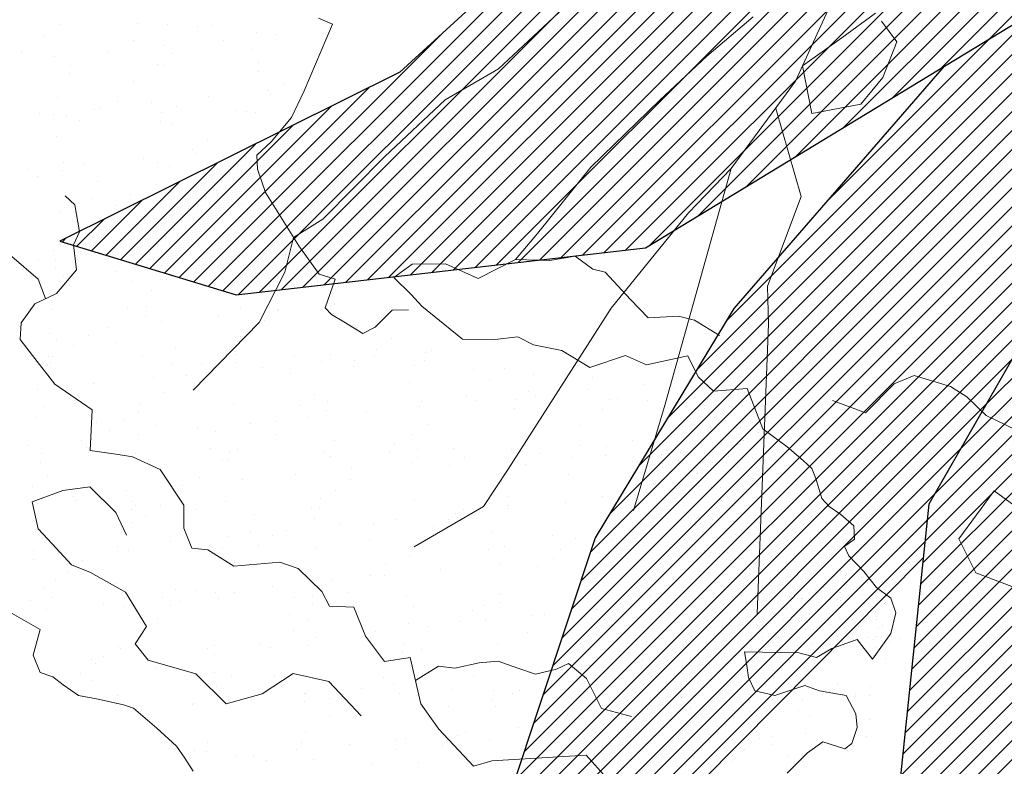
# Model space of a CAD drawing. Units: inches. Extents: x 1986 to 21484, y -1816 to 2016.
# Tile 55 of 85: x 3651.09 to 3662.33, y 1870.8 to 1879.32. Entities that reach past the tile are written whole.
import ezdxf

# ---------------------------------------------------------------- set-up
doc = ezdxf.new("R2010")
doc.units = ezdxf.units.IN
doc.layers.add('L-PLNT', color=84, linetype='Continuous', lineweight=13)
doc.layers.add('vfolhas', color=114, linetype='Continuous', lineweight=5)
for name, color, linetype in [('vfolha', 72, 'Continuous'), ('vfolha2', 110, 'Continuous'), ('vfolhas2', 102, 'Continuous')]:
    doc.layers.add(name, color=color, linetype=linetype)
pattern_1 = [(45, (-2446.5133113, 50.986076), (-0.004419417382, 0.004419417382), [])]

# ---------------------------------------------------------------- blocks, each defined once
blk = doc.blocks.new('arbusto_PB_verde_grande')
at = {"layer": 'vfolha2'}
h = blk.add_hatch(dxfattribs=at)
h.set_pattern_fill('ANSI31', color=256, scale=0.05, style=0)
h.set_pattern_definition(pattern_1)
h.paths.add_polyline_path([(0.02944, 0.35651), (0.00028, 0.09048), (0.02625, -0.03934), (0.047, 0.06233), (0.06189, 0.09731), (0.09372, 0.26573), (0.09955, 0.43473), (0.08789, 0.61313), (0.0645, 0.72266), (0.04988, 0.6851), (0.0236, 0.51294)])
h.paths.add_polyline_path([(0.30106, 0.43789), (0.14225, 0.24871), (0.26685, 0.30022)])
h.paths.add_polyline_path([(0.37995, 0.22817), (0.23697, 0.15193), (0.18428, 0.09364), (0.11122, 0.04358), (0.02625, -0.03934), (0.28061, 0.04667), (0.36829, 0.07798), (0.46756, 0.11239), (0.61068, 0.19376), (0.71585, 0.27823), (0.55813, 0.25948)])
h.paths.add_polyline_path([(0.56101, -0.29441), (0.72752, -0.32573), (0.59024, -0.2412), (0.42962, -0.15982), (0.02625, -0.03934), (0.14922, -0.14107), (0.18838, -0.16604), (0.41501, -0.24435)])
h.paths.add_polyline_path([(-0.27429, -0.44776), (-0.30352, -0.72628), (-0.23923, -0.64175), (-0.15457, -0.45716), (0.02625, -0.03934), (-0.16328, -0.25376)])
h.paths.add_polyline_path([(-0.51963, -0.24744), (-0.67736, -0.32573), (-0.59558, -0.35072), (-0.40574, -0.32882), (-0.21007, -0.20995), (0.02625, -0.03934), (-0.14874, -0.06595), (-0.31518, -0.09101), (-0.41452, -0.15048)])
h.paths.add_polyline_path([(-0.52546, 0.25007), (-0.70947, 0.24698), (-0.51963, 0.1093), (-0.32979, 0.02167), (-0.07567, -0.0128), (-0.04234, -0.02148), (-0.35024, 0.1312)])
at = {"layer": 'vfolhas'}
h = blk.add_hatch(dxfattribs=at)
h.set_pattern_fill('ANSI31', color=256, scale=0.05, style=0)
h.set_pattern_definition(pattern_1)
h.paths.add_polyline_path([(-0.57219, 0.06233), (-0.7153, 0.10298), (-0.67736, 0.08107), (-0.62769, 0.01536), (-0.56347, -0.04095), (-0.26461, -0.0834), (-0.14874, -0.06595), (-0.10151, -0.05877), (-0.20418, -0.0472), (-0.40279, -0.00339)])
h.paths.add_polyline_path([(-0.56347, -0.04095), (-0.58279, -0.02401), (-0.72992, -0.09726), (-0.4334, -0.1679), (-0.41452, -0.15048), (-0.31518, -0.09101), (-0.26461, -0.0834)])
h.paths.add_polyline_path([(-0.2769, -0.47267), (-0.27429, -0.44776), (-0.16328, -0.25376), (0.02625, -0.03934), (-0.21007, -0.20995), (-0.2672, -0.24466), (-0.36485, -0.35697), (-0.42907, -0.46341), (-0.47586, -0.60425), (-0.37946, -0.57603)])
at = {"layer": 'vfolha'}
blk.add_line((-0.2672, -0.24466), (-0.36485, -0.35697), dxfattribs=at)
at = {"layer": 'vfolha2'}
for p, q in [((-0.41452, -0.15048), (-0.51963, -0.24744)), ((-0.40574, -0.32882), (-0.21007, -0.20995)), ((-0.51963, -0.24744), (-0.67736, -0.32573)), ((-0.16328, -0.25376), (-0.27429, -0.44776)), ((-0.67736, -0.32573), (-0.59558, -0.35072)), ((-0.59558, -0.35072), (-0.40574, -0.32882)), ((-0.27429, -0.44776), (-0.30352, -0.72628))]:
    blk.add_line(p, q, dxfattribs=at)
at = {"layer": 'vfolhas2'}
for p, q in [((-0.36485, -0.35697), (-0.42907, -0.46341)), ((-0.42907, -0.46341), (-0.47586, -0.60425)), ((-0.37946, -0.57603), (-0.2769, -0.47267))]:
    blk.add_line(p, q, dxfattribs=at)
blk = doc.blocks.new('PLANT-SHRUB')
for p, q in [((2177.672, 1894.564), (2177.672, 1894.564)), ((2177.944, 1894.39), (2177.944, 1894.39)), ((2178.017, 1894.405), (2178.017, 1894.405)), ((2178.018, 1894.458), (2178.018, 1894.458)), ((2177.065, 1894.178), (2177.065, 1894.178)), ((2177.327, 1894.204), (2177.327, 1894.204)), ((2178.31, 1894.176), (2178.31, 1894.176)), ((2177.453, 1894.049), (2177.453, 1894.049)), ((2177.87, 1894.133), (2177.87, 1894.133)), ((2178.078, 1894.105), (2178.078, 1894.105)), ((2178.142, 1894.068), (2178.142, 1894.068)), ((2178.403, 1894.062), (2178.403, 1894.062)), ((2177.546, 1894.026), (2177.546, 1894.026)), ((2178.532, 1894.01), (2178.532, 1894.01)), ((2176.315, 1893.671), (2176.561, 1893.167)), ((2177.992, 1893.635), (2177.992, 1893.635)), ((2178.748, 1893.675), (2178.748, 1893.675)), ((2178.925, 1893.619), (2178.757, 1893.53)), ((2179.023, 1893.61), (2178.925, 1893.619)), ((2179.014, 1893.64), (2179.014, 1893.64)), ((2179.155, 1893.38), (2179.023, 1893.61)), ((2177.349, 1893.564), (2177.349, 1893.564)), ((2178.594, 1893.561), (2178.594, 1893.561)), ((2178.757, 1893.53), (2178.66, 1893.407)), ((2178.66, 1893.407), (2178.598, 1893.177)), ((2179.368, 1893.353), (2179.155, 1893.38)), ((2179.695, 1893.362), (2179.368, 1893.353)), ((2177.427, 1893.279), (2177.427, 1893.279)), ((2178.326, 1893.289), (2178.326, 1893.289)), ((2178.4, 1893.356), (2178.4, 1893.356)), ((2176.561, 1893.167), (2176.438, 1892.753)), ((2177.502, 1893.146), (2177.502, 1893.146)), ((2177.987, 1893.175), (2177.987, 1893.175)), ((2178.507, 1893.24), (2178.507, 1893.24)), ((2178.598, 1893.177), (2178.784, 1892.929)), ((2179.232, 1893.173), (2179.232, 1893.173)), ((2179.553, 1893.226), (2179.553, 1893.226)), ((2175.766, 1892.63), (2175.688, 1893.055)), ((2177.71, 1893.119), (2177.71, 1893.119)), ((2178.094, 1893.079), (2177.74, 1893.009)), ((2177.819, 1893.067), (2177.819, 1893.067)), ((2178.035, 1893.076), (2178.035, 1893.076)), ((2178.053, 1893.059), (2178.053, 1893.059)), ((2178.067, 1892.797), (2178.094, 1893.079)), ((2178.094, 1893.079), (2178.094, 1893.079)), ((2179.063, 1893.065), (2179.063, 1893.065)), ((2177.74, 1893.009), (2177.537, 1892.876)), ((2177.894, 1892.913), (2177.894, 1892.913)), ((2177.929, 1892.924), (2177.929, 1892.924)), ((2177.973, 1893.018), (2177.973, 1893.018)), ((2178.578, 1893.005), (2178.578, 1893.005)), ((2178.784, 1892.929), (2178.864, 1892.77)), ((2178.786, 1892.977), (2178.786, 1892.977)), ((2179.111, 1892.935), (2179.111, 1892.935)), ((2179.528, 1892.938), (2179.528, 1892.938)), ((2179.602, 1893.005), (2179.602, 1893.005)), ((2177.537, 1892.876), (2177.466, 1892.717)), ((2177.748, 1892.875), (2177.748, 1892.875)), ((2177.797, 1892.866), (2177.797, 1892.866)), ((2177.966, 1892.865), (2177.966, 1892.865)), ((2178.989, 1892.87), (2178.989, 1892.87)), ((2179.653, 1892.863), (2179.653, 1892.863)), ((2179.862, 1892.836), (2179.862, 1892.836)), ((2180.068, 1892.831), (2180.068, 1892.831)), ((2176.438, 1892.753), (2175.766, 1892.63)), ((2177.466, 1892.717), (2177.501, 1892.514)), ((2177.479, 1892.735), (2177.479, 1892.735)), ((2177.545, 1892.715), (2177.545, 1892.715)), ((2177.554, 1892.711), (2177.554, 1892.711)), ((2177.562, 1892.724), (2177.562, 1892.724)), ((2177.692, 1892.707), (2177.692, 1892.707)), ((2177.726, 1892.758), (2177.726, 1892.758)), ((2177.755, 1892.785), (2177.755, 1892.785)), ((2177.963, 1892.71), (2177.963, 1892.71)), ((2178.052, 1892.71), (2178.052, 1892.71)), ((2178.35, 1892.673), (2178.067, 1892.797)), ((2178.864, 1892.77), (2179.191, 1892.62)), ((2177.487, 1892.668), (2177.487, 1892.668)), ((2177.567, 1892.613), (2177.567, 1892.613)), ((2177.581, 1892.606), (2177.581, 1892.606)), ((2177.91, 1892.679), (2177.91, 1892.679)), ((2177.985, 1892.667), (2177.985, 1892.667)), ((2177.993, 1892.668), (2177.993, 1892.668)), ((2178.123, 1892.651), (2178.123, 1892.651)), ((2178.206, 1892.618), (2178.206, 1892.618)), ((2178.236, 1892.645), (2178.236, 1892.645)), ((2178.34, 1892.622), (2178.34, 1892.622)), ((2178.545, 1892.629), (2178.35, 1892.673)), ((2178.423, 1892.611), (2178.423, 1892.611)), ((2178.66, 1892.452), (2178.545, 1892.629)), ((2178.553, 1892.594), (2178.553, 1892.594)), ((2179.13, 1892.573), (2179.13, 1892.573)), ((2179.191, 1892.62), (2179.323, 1892.425)), ((2177.027, 1892.563), (2177.027, 1892.563)), ((2177.402, 1892.509), (2177.402, 1892.509)), ((2177.501, 1892.514), (2177.484, 1892.284)), ((2177.507, 1892.538), (2177.507, 1892.538)), ((2177.668, 1892.465), (2177.668, 1892.465)), ((2177.738, 1892.567), (2177.738, 1892.567)), ((2178.047, 1892.472), (2178.047, 1892.472)), ((2178.166, 1892.464), (2178.166, 1892.464)), ((2178.169, 1892.551), (2178.169, 1892.551)), ((2178.271, 1892.561), (2178.271, 1892.561)), ((2178.482, 1892.47), (2178.482, 1892.47)), ((2178.588, 1892.546), (2178.588, 1892.546)), ((2179.516, 1892.558), (2179.516, 1892.558)), ((2175.047, 1892.46), (2175.244, 1891.941)), ((2177.535, 1892.407), (2177.535, 1892.407)), ((2177.953, 1892.402), (2177.953, 1892.402)), ((2178.362, 1892.404), (2178.362, 1892.404)), ((2179.102, 1892.019), (2178.66, 1892.452)), ((2179.323, 1892.425), (2179.27, 1892.266)), ((2179.528, 1892.456), (2179.528, 1892.456)), ((2177.484, 1892.284), (2177.484, 1892.037)), ((2177.545, 1892.313), (2177.545, 1892.313)), ((2177.727, 1892.259), (2177.727, 1892.259)), ((2177.762, 1892.284), (2177.762, 1892.284)), ((2177.845, 1892.273), (2177.845, 1892.273)), ((2177.855, 1892.267), (2177.855, 1892.267)), ((2177.879, 1892.318), (2177.879, 1892.318)), ((2177.908, 1892.345), (2177.908, 1892.345)), ((2177.923, 1892.31), (2177.923, 1892.31)), ((2177.975, 1892.256), (2177.975, 1892.256)), ((2178.159, 1892.243), (2178.159, 1892.243)), ((2178.353, 1892.266), (2178.353, 1892.266)), ((2178.421, 1892.309), (2178.421, 1892.309)), ((2178.528, 1892.332), (2178.528, 1892.332)), ((2178.578, 1892.238), (2178.578, 1892.238)), ((2178.782, 1892.255), (2178.782, 1892.255)), ((2179.27, 1892.266), (2179.191, 1892.151)), ((2177.665, 1892.174), (2177.665, 1892.174)), ((2177.719, 1892.172), (2177.719, 1892.172)), ((2178.193, 1892.228), (2178.193, 1892.228)), ((2178.276, 1892.217), (2178.276, 1892.217)), ((2178.359, 1892.178), (2178.359, 1892.178)), ((2178.389, 1892.205), (2178.389, 1892.205)), ((2178.406, 1892.199), (2178.406, 1892.199)), ((2178.623, 1892.171), (2178.623, 1892.171)), ((2178.706, 1892.16), (2178.706, 1892.16)), ((2178.709, 1892.187), (2178.709, 1892.187)), ((2178.836, 1892.143), (2178.836, 1892.143)), ((2178.909, 1892.172), (2178.909, 1892.172)), ((2179.191, 1892.151), (2179.102, 1892.019)), ((2180.154, 1892.169), (2180.154, 1892.169)), ((2180.332, 1892.223), (2180.332, 1892.223)), ((2177.484, 1892.037), (2177.448, 1891.922)), ((2177.666, 1892.09), (2177.666, 1892.09)), ((2177.941, 1892.095), (2177.941, 1892.095)), ((2177.943, 1892.094), (2177.943, 1892.094)), ((2178.036, 1892.064), (2178.036, 1892.064)), ((2178.2, 1892.032), (2178.2, 1892.032)), ((2178.209, 1892.018), (2178.209, 1892.018)), ((2178.352, 1892.096), (2178.352, 1892.096)), ((2178.534, 1892.063), (2178.534, 1892.063)), ((2178.741, 1892.064), (2178.741, 1892.064)), ((2178.784, 1892.08), (2178.784, 1892.08)), ((2178.84, 1892.037), (2178.84, 1892.037)), ((2178.869, 1892.064), (2178.869, 1892.064)), ((2178.964, 1892.1), (2178.964, 1892.1)), ((2179.032, 1892.062), (2179.032, 1892.062)), ((2179.102, 1892.019), (2179.102, 1892.019)), ((2179.985, 1892.062), (2179.985, 1892.062)), ((2180.043, 1892.061), (2180.043, 1892.061)), ((2175.244, 1891.941), (2175.262, 1891.636)), ((2177.307, 1891.939), (2177.209, 1891.824)), ((2177.448, 1891.922), (2177.307, 1891.939)), ((2178.292, 1891.909), (2178.292, 1891.909)), ((2178.417, 1891.991), (2178.417, 1891.991)), ((2178.568, 1891.93), (2178.568, 1891.93)), ((2178.742, 1891.948), (2178.742, 1891.948)), ((2178.789, 1891.908), (2178.789, 1891.908)), ((2179.984, 1891.904), (2179.984, 1891.904)), ((2181.234, 1891.991), (2181.225, 1891.643)), ((2176.344, 1889.483), (2178.697, 1891.799)), ((2177.209, 1891.824), (2177.227, 1891.63)), ((2178.681, 1891.891), (2178.681, 1891.891)), ((2178.722, 1891.865), (2178.722, 1891.865)), ((2179.285, 1891.877), (2179.285, 1891.877)), ((2179.493, 1891.849), (2179.493, 1891.849)), ((2179.818, 1891.807), (2179.818, 1891.807)), ((2179.91, 1891.837), (2179.91, 1891.837)), ((2178.689, 1891.748), (2178.689, 1891.748)), ((2179.503, 1891.686), (2179.503, 1891.686)), ((2180.361, 1891.735), (2180.361, 1891.735)), ((2180.525, 1891.691), (2180.525, 1891.691)), ((2180.736, 1891.375), (2180.547, 1891.676)), ((2180.569, 1891.708), (2180.569, 1891.708)), ((2175.262, 1891.636), (2175.316, 1891.422)), ((2177.227, 1891.63), (2177.262, 1891.471)), ((2178.558, 1891.622), (2178.558, 1891.622)), ((2180.894, 1891.665), (2180.894, 1891.665)), ((2181.225, 1891.643), (2182.057, 1890.952)), ((2181.437, 1891.593), (2181.437, 1891.593)), ((2177.262, 1891.471), (2177.262, 1891.347)), ((2178.593, 1891.464), (2178.593, 1891.464)), ((2178.66, 1891.507), (2178.66, 1891.507)), ((2178.764, 1891.464), (2178.764, 1891.464)), ((2179.193, 1891.557), (2179.193, 1891.557)), ((2179.512, 1891.472), (2179.512, 1891.472)), ((2180.438, 1891.555), (2180.438, 1891.555)), ((2181.112, 1891.486), (2181.112, 1891.486)), ((2181.185, 1891.553), (2181.185, 1891.553)), ((2175.316, 1891.422), (2175.531, 1891.046)), ((2177.262, 1891.347), (2177.156, 1891.135)), ((2178.328, 1891.382), (2178.328, 1891.382)), ((2178.411, 1891.371), (2178.411, 1891.371)), ((2178.541, 1891.354), (2178.541, 1891.354)), ((2180.625, 1891.008), (2180.736, 1891.375)), ((2178.276, 1891.262), (2178.276, 1891.262)), ((2178.548, 1891.314), (2178.548, 1891.314)), ((2178.665, 1891.296), (2178.665, 1891.296)), ((2178.694, 1891.323), (2178.694, 1891.323)), ((2178.758, 1891.325), (2178.758, 1891.325)), ((2178.938, 1891.33), (2178.938, 1891.33)), ((2180.018, 1891.291), (2180.018, 1891.291)), ((2181.064, 1891.278), (2181.064, 1891.278)), ((2177.156, 1891.135), (2177.112, 1891.02)), ((2178.322, 1891.171), (2178.322, 1891.171)), ((2178.506, 1891.151), (2178.506, 1891.151)), ((2179.165, 1891.153), (2179.165, 1891.153)), ((2179.831, 1891.169), (2179.831, 1891.169)), ((2180.714, 1891.121), (2180.714, 1891.121)), ((2181.076, 1891.166), (2181.076, 1891.166)), ((2175.531, 1891.046), (2175.764, 1890.957)), ((2177.112, 1891.02), (2177.121, 1890.887)), ((2177.963, 1891.016), (2177.963, 1891.016)), ((2177.966, 1891.065), (2177.966, 1891.065)), ((2178.033, 1891.108), (2178.033, 1891.108)), ((2178.119, 1891.011), (2178.119, 1891.011)), ((2178.367, 1891.023), (2178.367, 1891.023)), ((2178.464, 1891.064), (2178.464, 1891.064)), ((2178.531, 1891.107), (2178.531, 1891.107)), ((2178.537, 1891.006), (2178.537, 1891.006)), ((2179.091, 1891.086), (2179.091, 1891.086)), ((2179.662, 1891.061), (2179.662, 1891.061)), ((2180.658, 1890.74), (2180.625, 1891.008)), ((2180.907, 1891.059), (2180.907, 1891.059)), ((2175.764, 1890.957), (2176.229, 1890.974)), ((2176.229, 1890.974), (2176.408, 1890.617)), ((2176.229, 1890.974), (2176.229, 1890.974)), ((2177.121, 1890.887), (2177.147, 1890.649)), ((2178.181, 1890.987), (2178.181, 1890.987)), ((2178.264, 1890.976), (2178.264, 1890.976)), ((2178.337, 1890.996), (2178.337, 1890.996)), ((2178.394, 1890.959), (2178.394, 1890.959)), ((2178.611, 1890.931), (2178.611, 1890.931)), ((2178.916, 1890.89), (2178.916, 1890.89)), ((2179.477, 1890.916), (2179.477, 1890.916)), ((2180.5, 1890.921), (2180.5, 1890.921)), ((2182.057, 1890.952), (2182.25, 1890.855)), ((2177.903, 1890.861), (2177.903, 1890.861)), ((2178.147, 1890.862), (2178.147, 1890.862)), ((2178.178, 1890.85), (2178.178, 1890.85)), ((2178.312, 1890.863), (2178.312, 1890.863)), ((2178.645, 1890.861), (2178.645, 1890.861)), ((2179.125, 1890.863), (2179.125, 1890.863)), ((2179.449, 1890.82), (2179.449, 1890.82)), ((2180.366, 1890.803), (2180.366, 1890.803)), ((2181.579, 1890.882), (2181.579, 1890.882)), ((2182.25, 1890.855), (2182.25, 1890.276)), ((2177.677, 1890.719), (2177.677, 1890.719)), ((2177.837, 1890.665), (2177.837, 1890.665)), ((2177.904, 1890.708), (2177.904, 1890.708)), ((2178.01, 1890.696), (2178.01, 1890.696)), ((2178.039, 1890.723), (2178.039, 1890.723)), ((2178.109, 1890.703), (2178.109, 1890.703)), ((2178.335, 1890.664), (2178.335, 1890.664)), ((2178.402, 1890.707), (2178.402, 1890.707)), ((2178.527, 1890.698), (2178.527, 1890.698)), ((2178.693, 1890.721), (2178.693, 1890.721)), ((2179.992, 1890.749), (2179.992, 1890.749)), ((2180.2, 1890.721), (2180.2, 1890.721)), ((2180.292, 1890.735), (2180.292, 1890.735)), ((2180.525, 1890.679), (2180.525, 1890.679)), ((2180.803, 1890.696), (2180.658, 1890.74)), ((2181.015, 1890.573), (2180.803, 1890.696)), ((2181.915, 1890.77), (2181.915, 1890.77)), ((2177.147, 1890.649), (2177.209, 1890.308)), ((2177.474, 1890.559), (2177.474, 1890.559)), ((2177.603, 1890.649), (2177.603, 1890.649)), ((2177.686, 1890.639), (2177.686, 1890.639)), ((2177.816, 1890.621), (2177.816, 1890.621)), ((2177.851, 1890.55), (2177.851, 1890.55)), ((2177.893, 1890.553), (2177.893, 1890.553)), ((2178.033, 1890.593), (2178.033, 1890.593)), ((2178.116, 1890.582), (2178.116, 1890.582)), ((2178.246, 1890.565), (2178.246, 1890.565)), ((2178.302, 1890.555), (2178.302, 1890.555)), ((2178.49, 1890.556), (2178.49, 1890.556)), ((2178.52, 1890.583), (2178.52, 1890.583)), ((2178.87, 1890.557), (2178.87, 1890.557)), ((2178.913, 1890.56), (2178.913, 1890.56)), ((2180.115, 1890.554), (2180.115, 1890.554)), ((2181.115, 1890.384), (2181.015, 1890.573)), ((2181.068, 1890.607), (2181.068, 1890.607)), ((2181.276, 1890.58), (2181.276, 1890.58)), ((2181.36, 1890.552), (2181.36, 1890.552)), ((2177.52, 1890.463), (2177.52, 1890.463)), ((2178.018, 1890.462), (2178.018, 1890.462)), ((2178.464, 1890.536), (2178.464, 1890.536)), ((2178.516, 1890.461), (2178.516, 1890.461)), ((2178.547, 1890.525), (2178.547, 1890.525)), ((2179.993, 1890.521), (2179.993, 1890.521)), ((2181.039, 1890.507), (2181.039, 1890.507)), ((2181.568, 1890.452), (2181.568, 1890.452)), ((2181.601, 1890.537), (2181.601, 1890.537)), ((2182.061, 1890.512), (2182.061, 1890.512)), ((2182.144, 1890.466), (2182.144, 1890.466)), ((2182.352, 1890.438), (2182.352, 1890.438)), ((2177.667, 1890.411), (2177.667, 1890.411)), ((2177.682, 1890.396), (2177.682, 1890.396)), ((2177.711, 1890.423), (2177.711, 1890.423)), ((2178.099, 1890.395), (2178.099, 1890.395)), ((2178.331, 1890.41), (2178.331, 1890.41)), ((2178.517, 1890.39), (2178.517, 1890.39)), ((2179.895, 1890.371), (2179.895, 1890.371)), ((2181.226, 1890.172), (2181.115, 1890.384)), ((2181.494, 1890.384), (2181.494, 1890.384)), ((2182.677, 1890.395), (2182.677, 1890.395)), ((2177.209, 1890.308), (2177.023, 1889.848)), ((2177.21, 1890.265), (2177.21, 1890.265)), ((2177.238, 1890.284), (2177.238, 1890.284)), ((2177.277, 1890.308), (2177.277, 1890.308)), ((2177.456, 1890.255), (2177.456, 1890.255)), ((2177.464, 1890.251), (2177.464, 1890.251)), ((2177.523, 1890.25), (2177.523, 1890.25)), ((2177.539, 1890.244), (2177.539, 1890.244)), ((2177.669, 1890.227), (2177.669, 1890.227)), ((2177.708, 1890.264), (2177.708, 1890.264)), ((2177.775, 1890.307), (2177.775, 1890.307)), ((2177.883, 1890.245), (2177.883, 1890.245)), ((2178.163, 1890.255), (2178.163, 1890.255)), ((2178.192, 1890.282), (2178.192, 1890.282)), ((2178.206, 1890.263), (2178.206, 1890.263)), ((2178.273, 1890.306), (2178.273, 1890.306)), ((2178.292, 1890.247), (2178.292, 1890.247)), ((2182.25, 1890.276), (2182.202, 1889.922)), ((2182.25, 1890.276), (2182.25, 1890.276)), ((2177.248, 1890.101), (2177.248, 1890.101)), ((2177.384, 1890.122), (2177.384, 1890.122)), ((2177.657, 1890.103), (2177.657, 1890.103)), ((2177.886, 1890.198), (2177.886, 1890.198)), ((2177.969, 1890.187), (2177.969, 1890.187)), ((2178.003, 1890.109), (2178.003, 1890.109)), ((2178.099, 1890.17), (2178.099, 1890.17)), ((2178.316, 1890.142), (2178.316, 1890.142)), ((2178.399, 1890.131), (2178.399, 1890.131)), ((2179.452, 1890.146), (2179.452, 1890.146)), ((2179.508, 1890.168), (2179.508, 1890.168)), ((2180.475, 1890.151), (2180.475, 1890.151)), ((2180.753, 1890.166), (2180.753, 1890.166)), ((2181.394, 1890.039), (2181.226, 1890.172)), ((2181.554, 1890.112), (2181.554, 1890.112)), ((2181.997, 1890.163), (2181.997, 1890.163)), ((2182.769, 1890.101), (2182.769, 1890.101)), ((2177.354, 1890.095), (2177.354, 1890.095)), ((2177.391, 1890.062), (2177.391, 1890.062)), ((2177.889, 1890.061), (2177.889, 1890.061)), ((2178.089, 1890.087), (2178.089, 1890.087)), ((2178.387, 1890.061), (2178.387, 1890.061)), ((2179.34, 1890.06), (2179.34, 1890.06)), ((2179.547, 1890.052), (2179.547, 1890.052)), ((2180.584, 1890.058), (2180.584, 1890.058)), ((2181.096, 1890.02), (2181.096, 1890.02)), ((2181.639, 1889.894), (2181.394, 1890.039)), ((2181.829, 1890.056), (2181.829, 1890.056)), ((2182.6, 1890.099), (2182.6, 1890.099)), ((2182.695, 1890.034), (2182.695, 1890.034)), ((2183.074, 1890.054), (2183.074, 1890.054)), ((2177.091, 1889.889), (2177.091, 1889.889)), ((2177.148, 1889.908), (2177.148, 1889.908)), ((2177.195, 1889.95), (2177.195, 1889.95)), ((2177.454, 1889.943), (2177.454, 1889.943)), ((2177.646, 1889.907), (2177.646, 1889.907)), ((2177.827, 1889.339), (2178.923, 1889.978)), ((2177.835, 1889.955), (2177.835, 1889.955)), ((2177.864, 1889.982), (2177.864, 1889.982)), ((2177.873, 1889.937), (2177.873, 1889.937)), ((2178.144, 1889.906), (2178.144, 1889.906)), ((2178.282, 1889.939), (2178.282, 1889.939)), ((2178.548, 1889.904), (2178.548, 1889.904)), ((2178.756, 1889.877), (2178.756, 1889.877)), ((2179.473, 1889.984), (2179.473, 1889.984)), ((2181.761, 1889.749), (2181.639, 1889.894)), ((2182.202, 1889.922), (2181.928, 1889.454)), ((2177.023, 1889.848), (2177.324, 1889.61)), ((2177.056, 1889.822), (2177.056, 1889.822)), ((2177.081, 1889.865), (2177.081, 1889.865)), ((2177.238, 1889.793), (2177.238, 1889.793)), ((2177.308, 1889.86), (2177.308, 1889.86)), ((2177.391, 1889.849), (2177.391, 1889.849)), ((2177.521, 1889.832), (2177.521, 1889.832)), ((2177.866, 1889.785), (2177.866, 1889.785)), ((2178.077, 1889.863), (2178.077, 1889.863)), ((2178.079, 1889.779), (2178.079, 1889.779)), ((2178.316, 1889.815), (2178.316, 1889.815)), ((2178.345, 1889.842), (2178.345, 1889.842)), ((2178.888, 1889.79), (2178.888, 1889.79)), ((2179.081, 1889.834), (2179.081, 1889.834)), ((2177.262, 1889.662), (2177.262, 1889.662)), ((2177.507, 1889.655), (2177.507, 1889.655)), ((2177.537, 1889.682), (2177.537, 1889.682)), ((2178.169, 1889.747), (2178.169, 1889.747)), ((2178.252, 1889.736), (2178.252, 1889.736)), ((2178.382, 1889.719), (2178.382, 1889.719)), ((2179.624, 1889.763), (2179.624, 1889.763)), ((2179.832, 1889.735), (2179.832, 1889.735)), ((2179.968, 1889.751), (2179.968, 1889.751)), ((2180.157, 1889.692), (2180.157, 1889.692)), ((2180.748, 1889.701), (2180.748, 1889.701)), ((2181.014, 1889.737), (2181.014, 1889.737)), ((2182.065, 1889.688), (2181.761, 1889.749)), ((2182.036, 1889.742), (2182.036, 1889.742)), ((2182.298, 1889.669), (2182.298, 1889.669)), ((2183.116, 1889.703), (2183.116, 1889.703)), ((2177.324, 1889.61), (2177.341, 1889.371)), ((2177.444, 1889.635), (2177.444, 1889.635)), ((2178.548, 1889.556), (2178.548, 1889.556)), ((2179.075, 1889.62), (2179.075, 1889.62)), ((2179.792, 1889.554), (2179.792, 1889.554)), ((2180.675, 1889.634), (2180.675, 1889.634)), ((2180.7, 1889.621), (2180.7, 1889.621)), ((2180.908, 1889.593), (2180.908, 1889.593)), ((2181.037, 1889.551), (2181.037, 1889.551)), ((2181.233, 1889.551), (2181.233, 1889.551)), ((2182.281, 1889.549), (2182.281, 1889.549)), ((2182.792, 1889.56), (2182.792, 1889.018)), ((2183.526, 1889.547), (2183.526, 1889.547)), ((2176.055, 1889.155), (2176.344, 1889.483)), ((2177.348, 1889.509), (2177.348, 1889.509)), ((2177.374, 1889.438), (2177.374, 1889.438)), ((2177.45, 1889.464), (2177.45, 1889.464)), ((2177.517, 1889.507), (2177.517, 1889.507)), ((2177.637, 1889.487), (2177.637, 1889.487)), ((2181.775, 1889.479), (2181.775, 1889.479)), ((2181.928, 1889.454), (2182.173, 1889.288)), ((2181.983, 1889.452), (2181.983, 1889.452)), ((2175.438, 1887.895), (2177.827, 1889.339)), ((2177.341, 1889.371), (2177.262, 1889.115)), ((2177.434, 1889.327), (2177.434, 1889.327)), ((2177.591, 1889.409), (2177.591, 1889.409)), ((2177.674, 1889.398), (2177.674, 1889.398)), ((2178.381, 1889.389), (2178.381, 1889.389)), ((2179.427, 1889.376), (2179.427, 1889.376)), ((2180.449, 1889.381), (2180.449, 1889.381)), ((2181.529, 1889.342), (2181.529, 1889.342)), ((2181.95, 1889.35), (2181.95, 1889.35)), ((2182.308, 1889.409), (2182.308, 1889.409)), ((2182.575, 1889.329), (2182.575, 1889.329)), ((2182.851, 1889.338), (2182.851, 1889.338)), ((2183.499, 1889.318), (2183.499, 1889.318)), ((2183.598, 1889.334), (2183.598, 1889.334)), ((2177.631, 1889.261), (2177.631, 1889.261)), ((2178.654, 1889.234), (2178.654, 1889.234)), ((2178.728, 1889.301), (2178.728, 1889.301)), ((2180.277, 1889.269), (2180.277, 1889.269)), ((2181.876, 1889.283), (2181.876, 1889.283)), ((2182.173, 1889.288), (2182.133, 1888.93)), ((2183.059, 1889.31), (2183.059, 1889.31)), ((2183.384, 1889.267), (2183.384, 1889.267)), ((2175.073, 1888.674), (2176.055, 1889.155)), ((2176.839, 1889.192), (2176.839, 1889.192)), ((2176.928, 1888.868), (2176.839, 1889.192)), ((2177.262, 1889.115), (2177.677, 1888.868)), ((2177.262, 1889.115), (2177.262, 1889.115)), ((2177.388, 1889.106), (2177.388, 1889.106)), ((2177.941, 1889.169), (2177.941, 1889.169)), ((2179.185, 1889.167), (2179.185, 1889.167)), ((2180.43, 1889.165), (2180.43, 1889.165)), ((2181.675, 1889.163), (2181.675, 1889.163)), ((2182.919, 1889.16), (2182.919, 1889.16)), ((2183.927, 1889.196), (2183.927, 1889.196)), ((2177.84, 1889.015), (2177.84, 1889.015)), ((2178.863, 1889.02), (2178.863, 1889.02)), ((2179.017, 1889.06), (2179.017, 1889.06)), ((2179.942, 1888.981), (2179.942, 1888.981)), ((2180.262, 1889.057), (2180.262, 1889.057)), ((2181.506, 1889.055), (2181.506, 1889.055)), ((2182.751, 1889.053), (2182.751, 1889.053)), ((2182.792, 1889.018), (2183.027, 1888.675)), ((2183.151, 1889), (2183.151, 1889)), ((2183.995, 1889.051), (2183.995, 1889.051)), ((2177.029, 1888.712), (2176.928, 1888.868)), ((2177.677, 1888.868), (2177.778, 1888.623)), ((2178.179, 1888.918), (2178.179, 1888.918)), ((2178.256, 1888.869), (2178.256, 1888.869)), ((2178.388, 1888.89), (2178.388, 1888.89)), ((2179.856, 1888.883), (2179.856, 1888.883)), ((2179.929, 1888.951), (2179.929, 1888.951)), ((2180.989, 1888.967), (2180.989, 1888.967)), ((2181.478, 1888.918), (2181.478, 1888.918)), ((2182.133, 1888.93), (2182.006, 1888.597)), ((2182.011, 1888.972), (2182.011, 1888.972)), ((2183.078, 1888.932), (2183.078, 1888.932)), ((2183.09, 1888.933), (2183.09, 1888.933)), ((2184.137, 1888.92), (2184.137, 1888.92)), ((2178.712, 1888.848), (2178.712, 1888.848)), ((2179.255, 1888.776), (2179.255, 1888.776)), ((2179.642, 1888.652), (2180.139, 1888.772)), ((2180.139, 1888.772), (2181.03, 1888.566)), ((2174.599, 1887.742), (2175.073, 1888.674)), ((2177.297, 1888.489), (2177.029, 1888.712)), ((2177.529, 1888.118), (2179.642, 1888.652)), ((2179.463, 1888.749), (2179.463, 1888.749)), ((2179.788, 1888.706), (2179.788, 1888.706)), ((2183.027, 1888.675), (2183.443, 1888.603)), ((2184.353, 1888.649), (2184.353, 1888.649)), ((2184.622, 1888.704), (2184.589, 1888.532)), ((2177.778, 1888.623), (2178.169, 1888.444)), ((2178.225, 1888.555), (2178.225, 1888.555)), ((2178.356, 1888.619), (2178.356, 1888.619)), ((2179.402, 1888.606), (2179.402, 1888.606)), ((2179.469, 1888.553), (2179.469, 1888.553)), ((2180.331, 1888.635), (2180.331, 1888.635)), ((2180.424, 1888.611), (2180.424, 1888.611)), ((2180.539, 1888.607), (2180.539, 1888.607)), ((2180.714, 1888.55), (2180.714, 1888.55)), ((2180.864, 1888.564), (2180.864, 1888.564)), ((2181.057, 1888.532), (2181.057, 1888.532)), ((2181.131, 1888.6), (2181.131, 1888.6)), ((2181.504, 1888.572), (2181.504, 1888.572)), ((2181.959, 1888.548), (2181.959, 1888.548)), ((2182.006, 1888.597), (2182.197, 1888.398)), ((2182.55, 1888.559), (2182.55, 1888.559)), ((2182.68, 1888.568), (2182.68, 1888.568)), ((2183.203, 1888.546), (2183.203, 1888.546)), ((2183.443, 1888.603), (2183.822, 1888.404)), ((2183.443, 1888.603), (2183.443, 1888.603)), ((2183.572, 1888.563), (2183.572, 1888.563)), ((2184.279, 1888.581), (2184.279, 1888.581)), ((2184.448, 1888.544), (2184.448, 1888.544)), ((2184.589, 1888.532), (2184.564, 1888.368)), ((2177.297, 1888.198), (2177.297, 1888.489)), ((2178.169, 1888.444), (2178.27, 1888.086)), ((2178.169, 1888.444), (2178.169, 1888.444)), ((2179.458, 1888.519), (2179.458, 1888.519)), ((2181.407, 1888.493), (2181.407, 1888.493)), ((2181.615, 1888.466), (2181.615, 1888.466)), ((2181.94, 1888.423), (2181.94, 1888.423)), ((2173.071, 1888.134), (2173.464, 1888.322)), ((2173.464, 1888.322), (2173.858, 1888.374)), ((2173.621, 1888.305), (2173.621, 1888.305)), ((2173.727, 1888.316), (2173.727, 1888.316)), ((2173.858, 1888.374), (2174.149, 1888.186)), ((2173.858, 1888.374), (2173.858, 1888.374)), ((2173.858, 1888.374), (2173.858, 1888.374)), ((2182.197, 1888.398), (2182.149, 1888.215)), ((2182.483, 1888.351), (2182.483, 1888.351)), ((2182.691, 1888.324), (2182.691, 1888.324)), ((2183.822, 1888.404), (2183.84, 1887.917)), ((2184.564, 1888.368), (2184.589, 1888.064)), ((2173.848, 1888.234), (2173.848, 1888.234)), ((2173.885, 1888.268), (2173.885, 1888.268)), ((2177.297, 1887.774), (2177.297, 1888.198)), ((2178.838, 1888.249), (2178.838, 1888.249)), ((2179.11, 1888.2), (2179.11, 1888.2)), ((2179.917, 1888.211), (2179.917, 1888.211)), ((2180.963, 1888.197), (2180.963, 1888.197)), ((2181.986, 1888.202), (2181.986, 1888.202)), ((2182.149, 1888.215), (2182.165, 1887.842)), ((2182.332, 1888.249), (2182.332, 1888.249)), ((2183.016, 1888.281), (2183.016, 1888.281)), ((2183.559, 1888.21), (2183.559, 1888.21)), ((2183.881, 1888.217), (2183.881, 1888.217)), ((2173.036, 1887.844), (2173.071, 1888.134)), ((2173.071, 1888.134), (2173.071, 1888.134)), ((2173.351, 1888.118), (2173.351, 1888.118)), ((2173.423, 1888.123), (2173.423, 1888.123)), ((2173.862, 1888.12), (2173.862, 1888.12)), ((2174.046, 1888.122), (2174.046, 1888.122)), ((2174.149, 1888.186), (2174.337, 1888.066)), ((2176.141, 1887.929), (2177.529, 1888.118)), ((2178.27, 1888.086), (2178.46, 1887.818)), ((2178.863, 1888.166), (2178.863, 1888.166)), ((2179.036, 1888.132), (2179.036, 1888.132)), ((2180.107, 1888.164), (2180.107, 1888.164)), ((2180.659, 1888.168), (2180.659, 1888.168)), ((2181.352, 1888.162), (2181.352, 1888.162)), ((2182.258, 1888.182), (2182.258, 1888.182)), ((2182.597, 1888.159), (2182.597, 1888.159)), ((2183.065, 1888.163), (2183.065, 1888.163)), ((2183.767, 1888.182), (2183.767, 1888.182)), ((2183.841, 1888.157), (2183.841, 1888.157)), ((2184.092, 1888.14), (2184.092, 1888.14)), ((2184.111, 1888.15), (2184.111, 1888.15)), ((2173.156, 1888.027), (2173.156, 1888.027)), ((2173.339, 1888.069), (2173.339, 1888.069)), ((2173.427, 1887.991), (2173.427, 1887.991)), ((2173.531, 1887.978), (2173.531, 1887.978)), ((2173.649, 1888.052), (2173.649, 1888.052)), ((2173.961, 1888.068), (2173.961, 1888.068)), ((2174.337, 1888.066), (2174.043, 1887.599)), ((2174.337, 1888.066), (2174.337, 1888.066)), ((2178.694, 1888.059), (2178.694, 1888.059)), ((2179.939, 1888.057), (2179.939, 1888.057)), ((2181.183, 1888.054), (2181.183, 1888.054)), ((2182.428, 1888.052), (2182.428, 1888.052)), ((2183.673, 1888.05), (2183.673, 1888.05)), ((2184.589, 1888.064), (2184.626, 1887.716)), ((2173.069, 1887.94), (2173.069, 1887.94)), ((2173.439, 1887.859), (2173.439, 1887.859)), ((2173.475, 1887.893), (2173.475, 1887.893)), ((2173.609, 1887.92), (2173.609, 1887.92)), ((2173.694, 1887.956), (2173.694, 1887.956)), ((2173.965, 1887.92), (2173.965, 1887.92)), ((2174.069, 1887.907), (2174.069, 1887.907)), ((2174.132, 1887.913), (2174.132, 1887.913)), ((2174.221, 1887.672), (2175.438, 1887.895)), ((2175.438, 1887.895), (2176.141, 1887.929)), ((2183.534, 1887.898), (2183.534, 1887.898)), ((2183.84, 1887.917), (2184.129, 1887.429)), ((2173.565, 1887.816), (2173.565, 1887.816)), ((2177.375, 1887.651), (2177.297, 1887.774)), ((2178.46, 1887.818), (2178.527, 1887.628)), ((2178.887, 1887.79), (2178.887, 1887.79)), ((2179.095, 1887.763), (2179.095, 1887.763)), ((2179.377, 1887.836), (2179.377, 1887.836)), ((2180.238, 1887.782), (2180.238, 1887.782)), ((2180.311, 1887.849), (2180.311, 1887.849)), ((2180.399, 1887.841), (2180.399, 1887.841)), ((2181.479, 1887.802), (2181.479, 1887.802)), ((2181.861, 1887.817), (2181.861, 1887.817)), ((2182.165, 1887.842), (2182.269, 1887.643)), ((2182.525, 1887.788), (2182.525, 1887.788)), ((2183.46, 1887.831), (2183.46, 1887.831)), ((2183.547, 1887.793), (2183.547, 1887.793)), ((2184.627, 1887.755), (2184.627, 1887.755)), ((2172.884, 1887.124), (2174.221, 1887.672)), ((2173.498, 1887.673), (2173.023, 1887.729)), ((2173.338, 1887.733), (2173.338, 1887.733)), ((2174.043, 1887.599), (2173.498, 1887.673)), ((2173.849, 1887.735), (2173.849, 1887.735)), ((2174.039, 1887.684), (2174.039, 1887.684)), ((2174.076, 1887.717), (2174.076, 1887.717)), ((2177.42, 1887.405), (2177.375, 1887.651)), ((2178.527, 1887.628), (2178.739, 1887.472)), ((2179.42, 1887.72), (2179.42, 1887.72)), ((2179.963, 1887.648), (2179.963, 1887.648)), ((2182.269, 1887.643), (2182.682, 1887.317)), ((2184.626, 1887.716), (2184.684, 1887.612)), ((2173.884, 1887.621), (2173.884, 1887.621)), ((2179.147, 1887.552), (2179.147, 1887.552)), ((2180.171, 1887.621), (2180.171, 1887.621)), ((2180.391, 1887.55), (2180.391, 1887.55)), ((2180.496, 1887.578), (2180.496, 1887.578)), ((2181.636, 1887.547), (2181.636, 1887.547)), ((2182.88, 1887.545), (2182.88, 1887.545)), ((2184.125, 1887.543), (2184.125, 1887.543)), ((2184.684, 1887.612), (2184.851, 1887.364)), ((2184.735, 1887.547), (2184.735, 1887.547)), ((2177.667, 1887.245), (2177.42, 1887.405)), ((2178.739, 1887.472), (2179.007, 1887.215)), ((2179.84, 1887.417), (2179.84, 1887.417)), ((2179.892, 1887.44), (2179.892, 1887.44)), ((2180.938, 1887.427), (2180.938, 1887.427)), ((2181.038, 1887.507), (2181.038, 1887.507)), ((2181.247, 1887.479), (2181.247, 1887.479)), ((2181.439, 1887.431), (2181.439, 1887.431)), ((2181.513, 1887.498), (2181.513, 1887.498)), ((2181.571, 1887.436), (2181.571, 1887.436)), ((2181.961, 1887.432), (2181.961, 1887.432)), ((2183.062, 1887.466), (2183.062, 1887.466)), ((2184.129, 1887.429), (2184.111, 1887.195)), ((2184.661, 1887.48), (2184.661, 1887.48)), ((2182.114, 1887.365), (2182.114, 1887.365)), ((2182.322, 1887.338), (2182.322, 1887.338)), ((2182.647, 1887.295), (2182.647, 1887.295)), ((2182.682, 1887.317), (2182.772, 1886.981)), ((2182.682, 1887.317), (2182.682, 1887.317)), ((2183.04, 1887.393), (2183.04, 1887.393)), ((2184.086, 1887.38), (2184.086, 1887.38)), ((2184.851, 1887.364), (2184.984, 1887.18)), ((2177.945, 1886.966), (2177.667, 1887.245)), ((2179.007, 1887.215), (2179.086, 1886.623)), ((2183.19, 1887.223), (2183.19, 1887.223)), ((2183.398, 1887.196), (2183.398, 1887.196)), ((2184.111, 1887.195), (2183.88, 1887.136)), ((2184.984, 1887.18), (2185.03, 1886.972)), ((2179.492, 1887.099), (2179.492, 1887.099)), ((2179.784, 1887.163), (2179.784, 1887.163)), ((2180.374, 1887.071), (2180.374, 1887.071)), ((2181.029, 1887.161), (2181.029, 1887.161)), ((2182.274, 1887.159), (2182.274, 1887.159)), ((2182.641, 1887.08), (2182.641, 1887.08)), ((2182.714, 1887.148), (2182.714, 1887.148)), ((2183.518, 1887.156), (2183.518, 1887.156)), ((2183.723, 1887.153), (2183.723, 1887.153)), ((2183.88, 1887.136), (2183.785, 1886.689)), ((2184.264, 1887.115), (2184.264, 1887.115)), ((2184.266, 1887.082), (2184.266, 1887.082)), ((2184.763, 1887.154), (2184.763, 1887.154)), ((2177.558, 1886.922), (2177.945, 1886.966)), ((2178.404, 1886.835), (2177.945, 1886.966)), ((2179.352, 1887.066), (2179.352, 1887.066)), ((2179.419, 1887.031), (2179.419, 1887.031)), ((2179.616, 1887.056), (2179.616, 1887.056)), ((2180.861, 1887.054), (2180.861, 1887.054)), ((2181.041, 1887.066), (2181.041, 1887.066)), ((2181.453, 1887.032), (2181.453, 1887.032)), ((2182.105, 1887.051), (2182.105, 1887.051)), ((2182.5, 1887.018), (2182.5, 1887.018)), ((2182.772, 1886.981), (2182.892, 1886.841)), ((2183.35, 1887.049), (2183.35, 1887.049)), ((2183.522, 1887.023), (2183.522, 1887.023)), ((2184.474, 1887.054), (2184.474, 1887.054)), ((2184.594, 1887.047), (2184.594, 1887.047)), ((2184.601, 1886.984), (2184.601, 1886.984)), ((2184.799, 1887.012), (2184.799, 1887.012)), ((2185.03, 1886.972), (2185.053, 1886.823)), ((2176.595, 1886.787), (2177.558, 1886.922)), ((2174.071, 1886.806), (2174.764, 1886.768)), ((2174.764, 1886.768), (2175.497, 1886.768)), ((2175.497, 1886.768), (2176.595, 1886.787)), ((2178.56, 1886.456), (2178.404, 1886.835)), ((2180.694, 1886.748), (2180.694, 1886.748)), ((2182.892, 1886.841), (2182.802, 1886.61)), ((2182.892, 1886.841), (2182.892, 1886.841)), ((2183.916, 1886.797), (2183.916, 1886.797)), ((2185.053, 1886.823), (2185.122, 1886.69)), ((2179.086, 1886.623), (2179.086, 1886.444)), ((2179.594, 1886.662), (2179.594, 1886.662)), ((2179.802, 1886.635), (2179.802, 1886.635)), ((2179.867, 1886.67), (2179.867, 1886.67)), ((2180.62, 1886.68), (2180.62, 1886.68)), ((2180.913, 1886.657), (2180.913, 1886.657)), ((2181.935, 1886.662), (2181.935, 1886.662)), ((2182.243, 1886.716), (2182.243, 1886.716)), ((2183.015, 1886.623), (2183.015, 1886.623)), ((2183.785, 1886.689), (2183.926, 1886.251)), ((2183.785, 1886.689), (2183.785, 1886.689)), ((2183.842, 1886.729), (2183.842, 1886.729)), ((2185.122, 1886.69), (2185.047, 1886.494)), ((2179.227, 1886.548), (2179.368, 1886.425)), ((2180.068, 1886.549), (2180.068, 1886.549)), ((2180.127, 1886.592), (2180.127, 1886.592)), ((2180.67, 1886.52), (2180.67, 1886.52)), ((2181.313, 1886.547), (2181.313, 1886.547)), ((2182.558, 1886.544), (2182.558, 1886.544)), ((2182.802, 1886.61), (2182.621, 1886.419)), ((2183.802, 1886.542), (2183.802, 1886.542)), ((2184.061, 1886.61), (2184.061, 1886.61)), ((2178.84, 1886.199), (2178.56, 1886.456)), ((2179.086, 1886.444), (2179.097, 1886.165)), ((2179.368, 1886.425), (2179.641, 1886.434)), ((2179.641, 1886.434), (2179.79, 1886.39)), ((2180.878, 1886.493), (2180.878, 1886.493)), ((2181.203, 1886.45), (2181.203, 1886.45)), ((2181.895, 1886.397), (2181.895, 1886.397)), ((2182.621, 1886.419), (2182.54, 1885.937)), ((2185.047, 1886.494), (2184.788, 1886.333)), ((2179.79, 1886.39), (2179.86, 1886.144)), ((2180.222, 1886.316), (2180.222, 1886.316)), ((2180.349, 1886.301), (2180.349, 1886.301)), ((2181.746, 1886.379), (2181.746, 1886.379)), ((2181.822, 1886.329), (2181.822, 1886.329)), ((2181.954, 1886.351), (2181.954, 1886.351)), ((2182.279, 1886.309), (2182.279, 1886.309)), ((2183.444, 1886.365), (2183.444, 1886.365)), ((2184.788, 1886.333), (2184.967, 1885.753)), ((2184.788, 1886.333), (2184.788, 1886.333)), ((2179.097, 1886.165), (2178.84, 1886.199)), ((2181.428, 1886.262), (2181.428, 1886.262)), ((2182.474, 1886.248), (2182.474, 1886.248)), ((2182.822, 1886.237), (2182.822, 1886.237)), ((2183.03, 1886.21), (2183.03, 1886.21)), ((2183.244, 1885.949), (2183.334, 1886.22)), ((2183.497, 1886.253), (2183.497, 1886.253)), ((2183.926, 1886.251), (2184.021, 1886.039)), ((2184.576, 1886.214), (2184.576, 1886.214)), ((2179.097, 1886.165), (2179.097, 1886.165)), ((2179.86, 1886.144), (2179.904, 1885.986)), ((2180.706, 1886.16), (2180.706, 1886.16)), ((2181.951, 1886.158), (2181.951, 1886.158)), ((2183.196, 1886.156), (2183.196, 1886.156)), ((2183.355, 1886.167), (2183.355, 1886.167)), ((2183.897, 1886.095), (2183.897, 1886.095)), ((2184.105, 1886.068), (2184.105, 1886.068)), ((2184.44, 1886.153), (2184.44, 1886.153)), ((2179.875, 1885.997), (2179.875, 1885.997)), ((2179.904, 1885.986), (2179.904, 1885.881)), ((2180.538, 1886.053), (2180.538, 1886.053)), ((2181.424, 1885.965), (2181.424, 1885.965)), ((2181.782, 1886.05), (2181.782, 1886.05)), ((2183.023, 1885.979), (2183.023, 1885.979)), ((2183.027, 1886.048), (2183.027, 1886.048)), ((2183.097, 1886.046), (2183.097, 1886.046)), ((2183.262, 1885.534), (2183.244, 1885.949)), ((2184.021, 1886.039), (2184.021, 1885.714)), ((2184.272, 1886.046), (2184.272, 1886.046)), ((2184.43, 1886.025), (2184.43, 1886.025)), ((2184.646, 1886.014), (2184.646, 1886.014)), ((2179.904, 1885.881), (2179.597, 1885.722)), ((2179.801, 1885.93), (2179.801, 1885.93)), ((2179.842, 1885.9), (2179.842, 1885.9)), ((2180.888, 1885.887), (2180.888, 1885.887)), ((2181.91, 1885.892), (2181.91, 1885.892)), ((2182.54, 1885.937), (2182.671, 1885.616)), ((2182.99, 1885.853), (2182.99, 1885.853)), ((2184.036, 1885.84), (2184.036, 1885.84)), ((2179.597, 1885.722), (2179.693, 1885.555)), ((2181.076, 1885.646), (2181.076, 1885.646)), ((2182.625, 1885.614), (2182.625, 1885.614)), ((2182.671, 1885.616), (2182.772, 1885.485)), ((2184.021, 1885.714), (2184.021, 1885.479)), ((2184.224, 1885.628), (2184.224, 1885.628)), ((2184.298, 1885.695), (2184.298, 1885.695)), ((2179.693, 1885.555), (2179.641, 1885.16)), ((2179.746, 1885.548), (2179.746, 1885.548)), ((2179.759, 1885.606), (2179.759, 1885.606)), ((2180.301, 1885.534), (2180.301, 1885.534)), ((2180.324, 1885.53), (2180.324, 1885.53)), ((2180.51, 1885.507), (2180.51, 1885.507)), ((2180.568, 1885.489), (2181.646, 1885.537)), ((2180.99, 1885.546), (2180.99, 1885.546)), ((2181.002, 1885.579), (2181.002, 1885.579)), ((2182.235, 1885.544), (2182.235, 1885.544)), ((2183.515, 1885.353), (2183.262, 1885.534)), ((2183.48, 1885.541), (2183.48, 1885.541)), ((2179.962, 1885.271), (2180.568, 1885.489)), ((2180.834, 1885.464), (2180.834, 1885.464)), ((2181.377, 1885.392), (2181.377, 1885.392)), ((2181.403, 1885.492), (2181.403, 1885.492)), ((2182.449, 1885.478), (2182.449, 1885.478)), ((2182.772, 1885.485), (2182.973, 1885.234)), ((2183.472, 1885.483), (2183.472, 1885.483)), ((2184.021, 1885.479), (2183.858, 1885.209)), ((2179.618, 1885.049), (2179.962, 1885.271)), ((2181.585, 1885.365), (2181.585, 1885.365)), ((2181.91, 1885.322), (2181.91, 1885.322)), ((2182.278, 1885.296), (2182.278, 1885.296)), ((2183.858, 1885.209), (2183.515, 1885.353)), ((2175.422, 1885.249), (2176.598, 1885.249)), ((2176.598, 1885.249), (2177.283, 1885.089)), ((2179.641, 1885.16), (2179.5, 1884.457)), ((2180.384, 1885.159), (2180.384, 1885.159)), ((2180.605, 1885.214), (2180.605, 1885.214)), ((2181.628, 1885.157), (2181.628, 1885.157)), ((2182.204, 1885.228), (2182.204, 1885.228)), ((2182.453, 1885.251), (2182.453, 1885.251)), ((2182.973, 1885.234), (2182.641, 1884.913)), ((2182.661, 1885.223), (2182.661, 1885.223)), ((2182.986, 1885.181), (2182.986, 1885.181)), ((2183.827, 1885.263), (2183.827, 1885.263)), ((2183.858, 1885.209), (2183.858, 1885.209)), ((2177.283, 1885.089), (2178.228, 1885.089)), ((2178.228, 1885.089), (2179.234, 1885.126)), ((2179.234, 1885.126), (2179.618, 1885.049)), ((2179.816, 1885.13), (2179.816, 1885.13)), ((2180.215, 1885.052), (2180.215, 1885.052)), ((2180.863, 1885.117), (2180.863, 1885.117)), ((2181.46, 1885.05), (2181.46, 1885.05)), ((2181.885, 1885.122), (2181.885, 1885.122)), ((2182.704, 1885.047), (2182.704, 1885.047)), ((2182.873, 1885.155), (2182.873, 1885.155)), ((2182.965, 1885.083), (2182.965, 1885.083)), ((2183.529, 1885.109), (2183.529, 1885.109)), ((2183.737, 1885.082), (2183.737, 1885.082)), ((2183.479, 1884.945), (2183.479, 1884.945)), ((2180.183, 1884.828), (2180.183, 1884.828)), ((2180.257, 1884.896), (2180.257, 1884.896)), ((2181.806, 1884.864), (2181.806, 1884.864)), ((2182.641, 1884.913), (2182.752, 1884.406)), ((2183.405, 1884.877), (2183.405, 1884.877)), ((2178.584, 1884.814), (2178.584, 1884.814)), ((2179.276, 1884.755), (2179.276, 1884.755)), ((2180.298, 1884.76), (2180.298, 1884.76)), ((2181.378, 1884.721), (2181.378, 1884.721)), ((2182.424, 1884.708), (2182.424, 1884.708)), ((2183.446, 1884.713), (2183.446, 1884.713)), ((2178.857, 1884.689), (2178.857, 1884.689)), ((2179.065, 1884.662), (2179.065, 1884.662)), ((2179.39, 1884.619), (2179.39, 1884.619)), ((2179.423, 1884.547), (2179.423, 1884.547)), ((2179.933, 1884.548), (2179.933, 1884.548)), ((2180.141, 1884.52), (2180.141, 1884.52)), ((2180.668, 1884.545), (2180.668, 1884.545)), ((2181.458, 1884.545), (2181.458, 1884.545)), ((2181.912, 1884.543), (2181.912, 1884.543)), ((2183.007, 1884.513), (2183.007, 1884.513)), ((2183.157, 1884.54), (2183.157, 1884.54)), ((2178.712, 1884.399), (2178.712, 1884.399)), ((2179.5, 1884.457), (2179.386, 1884.202)), ((2179.785, 1884.464), (2179.785, 1884.464)), ((2180.466, 1884.478), (2180.466, 1884.478)), ((2181.009, 1884.406), (2181.009, 1884.406)), ((2181.217, 1884.379), (2181.217, 1884.379)), ((2181.385, 1884.477), (2181.385, 1884.477)), ((2182.752, 1884.406), (2182.712, 1883.995)), ((2182.752, 1884.406), (2182.752, 1884.406)), ((2179.791, 1884.36), (2179.791, 1884.36)), ((2180.837, 1884.347), (2180.837, 1884.347)), ((2181.542, 1884.336), (2181.542, 1884.336)), ((2181.86, 1884.352), (2181.86, 1884.352)), ((2182.085, 1884.265), (2182.085, 1884.265)), ((2182.939, 1884.313), (2182.939, 1884.313)), ((2178.816, 1884.161), (2178.816, 1884.161)), ((2179.386, 1884.202), (2179.28, 1884.079)), ((2179.438, 1884.145), (2179.438, 1884.145)), ((2180.061, 1884.158), (2180.061, 1884.158)), ((2181.305, 1884.156), (2181.305, 1884.156)), ((2182.293, 1884.237), (2182.293, 1884.237)), ((2182.55, 1884.154), (2182.55, 1884.154)), ((2182.618, 1884.194), (2182.618, 1884.194)), ((2182.66, 1884.194), (2182.66, 1884.194)), ((2178.7, 1884.036), (2178.383, 1883.913)), ((2178.648, 1884.053), (2178.648, 1884.053)), ((2179.06, 1884.079), (2178.7, 1884.036)), ((2179.28, 1884.079), (2179.06, 1884.079)), ((2179.364, 1884.078), (2179.364, 1884.078)), ((2179.892, 1884.051), (2179.892, 1884.051)), ((2180.987, 1884.113), (2180.987, 1884.113)), ((2181.137, 1884.049), (2181.137, 1884.049)), ((2182.381, 1884.047), (2182.381, 1884.047)), ((2182.586, 1884.127), (2182.586, 1884.127)), ((2179.251, 1883.985), (2179.251, 1883.985)), ((2180.273, 1883.99), (2180.273, 1883.99)), ((2181.353, 1883.951), (2181.353, 1883.951)), ((2182.399, 1883.938), (2182.399, 1883.938)), ((2182.712, 1883.995), (2182.692, 1883.764)), ((2178.383, 1883.913), (2177.627, 1883.579)), ((2178.489, 1883.703), (2178.489, 1883.703)), ((2178.966, 1883.713), (2178.966, 1883.713)), ((2180.565, 1883.727), (2180.565, 1883.727)), ((2180.639, 1883.794), (2180.639, 1883.794)), ((2182.188, 1883.762), (2182.188, 1883.762)), ((2182.692, 1883.764), (2182.551, 1883.633)), ((2178.687, 1883.629), (2178.687, 1883.629)), ((2178.697, 1883.676), (2178.697, 1883.676)), ((2179.022, 1883.633), (2179.022, 1883.633)), ((2179.766, 1883.59), (2179.766, 1883.59)), ((2181.677, 1883.623), (2181.506, 1883.392)), ((2182.029, 1883.663), (2181.677, 1883.623)), ((2181.677, 1883.623), (2181.677, 1883.623)), ((2182.29, 1883.583), (2182.029, 1883.663)), ((2182.159, 1883.623), (2182.068, 1883.402)), ((2182.551, 1883.633), (2182.29, 1883.583)), ((2177.627, 1883.579), (2177.697, 1883.42)), ((2179.1, 1883.546), (2179.1, 1883.546)), ((2179.564, 1883.561), (2179.564, 1883.561)), ((2179.773, 1883.534), (2179.773, 1883.534)), ((2180.097, 1883.491), (2180.097, 1883.491)), ((2180.345, 1883.544), (2180.345, 1883.544)), ((2180.812, 1883.577), (2180.812, 1883.577)), ((2181.589, 1883.542), (2181.589, 1883.542)), ((2181.835, 1883.582), (2181.835, 1883.582)), ((2178.619, 1883.394), (2178.619, 1883.394)), ((2180.168, 1883.362), (2180.168, 1883.362)), ((2180.64, 1883.42), (2180.64, 1883.42)), ((2180.848, 1883.392), (2180.848, 1883.392)), ((2181.506, 1883.392), (2181.355, 1883.332)), ((2181.767, 1883.376), (2181.767, 1883.376)), ((2181.841, 1883.443), (2181.841, 1883.443)), ((2182.068, 1883.402), (2182.113, 1883.009)), ((2178.545, 1883.327), (2178.545, 1883.327)), ((2181.173, 1883.35), (2181.173, 1883.35)), ((2181.355, 1883.332), (2181.184, 1883.071)), ((2181.355, 1883.332), (2181.355, 1883.332)), ((2181.716, 1883.278), (2181.716, 1883.278)), ((2181.924, 1883.251), (2181.924, 1883.251)), ((2178.179, 1883.229), (2178.179, 1883.229)), ((2178.493, 1883.16), (2178.493, 1883.16)), ((2179.226, 1883.215), (2179.226, 1883.215)), ((2179.738, 1883.158), (2179.738, 1883.158)), ((2180.248, 1883.22), (2180.248, 1883.22)), ((2180.983, 1883.155), (2180.983, 1883.155)), ((2181.328, 1883.181), (2181.328, 1883.181)), ((2178.325, 1883.052), (2178.325, 1883.052)), ((2179.569, 1883.05), (2179.569, 1883.05)), ((2179.82, 1883.044), (2179.82, 1883.044)), ((2180.814, 1883.048), (2180.814, 1883.048)), ((2181.184, 1883.071), (2181.194, 1882.92)), ((2179.746, 1882.976), (2179.746, 1882.976)), ((2181.369, 1883.011), (2181.369, 1883.011)), ((2178.661, 1882.859), (2178.661, 1882.859)), ((2179.741, 1882.82), (2179.741, 1882.82)), ((2180.787, 1882.807), (2180.787, 1882.807)), ((2181.021, 1882.693), (2181.021, 1882.693)), ((2178.653, 1882.647), (2178.653, 1882.647)), ((2179.196, 1882.575), (2179.196, 1882.575)), ((2179.348, 1882.612), (2179.348, 1882.612)), ((2180.948, 1882.625), (2180.948, 1882.625)), ((2178.777, 1882.546), (2178.777, 1882.546)), ((2179.404, 1882.548), (2179.404, 1882.548)), ((2179.729, 1882.505), (2179.729, 1882.505)), ((2180.022, 1882.543), (2180.022, 1882.543)), ((2181.267, 1882.541), (2181.267, 1882.541)), ((2179.201, 1882.445), (2179.201, 1882.445)), ((2180.223, 1882.45), (2180.223, 1882.45)), ((2180.272, 1882.434), (2180.272, 1882.434)), ((2180.48, 1882.406), (2180.48, 1882.406)), ((2180.805, 1882.363), (2180.805, 1882.363)), ((2181.302, 1882.411), (2181.302, 1882.411)), ((2179.001, 1882.293), (2179.001, 1882.293)), ((2180.55, 1882.261), (2180.55, 1882.261)), ((2179.415, 1882.157), (2179.415, 1882.157)), ((2180.66, 1882.155), (2180.66, 1882.155)), ((2179.247, 1882.049), (2179.247, 1882.049)), ((2179.716, 1882.05), (2179.716, 1882.05)), ((2180.491, 1882.047), (2180.491, 1882.047)), ((2180.762, 1882.036), (2180.762, 1882.036)), ((2180.202, 1881.942), (2180.202, 1881.942)), ((2180.129, 1881.875), (2180.129, 1881.875)), ((2180.198, 1881.68), (2180.198, 1881.68)), ((2179.903, 1881.447), (2179.903, 1881.447)), ((2180.111, 1881.42), (2180.111, 1881.42)), ((2180.436, 1881.377), (2180.436, 1881.377))]:
    blk.add_line(p, q)

msp = doc.modelspace()

# ---------------------------------------------------------------- block references
at = {"layer": 'L-PLNT', "rotation": 223.1883365522388}
msp.add_blockref('PLANT-SHRUB', (3953.27, 4742.965), dxfattribs=at)
at = {"layer": 'L-PLNT', "xscale": 24.60366729364114, "yscale": 24.60366729364114, "zscale": 24.60366729364114}
msp.add_blockref('arbusto_PB_verde_grande', (3668.218, 1884.805), dxfattribs=at)

doc.saveas('drawing.dxf')
